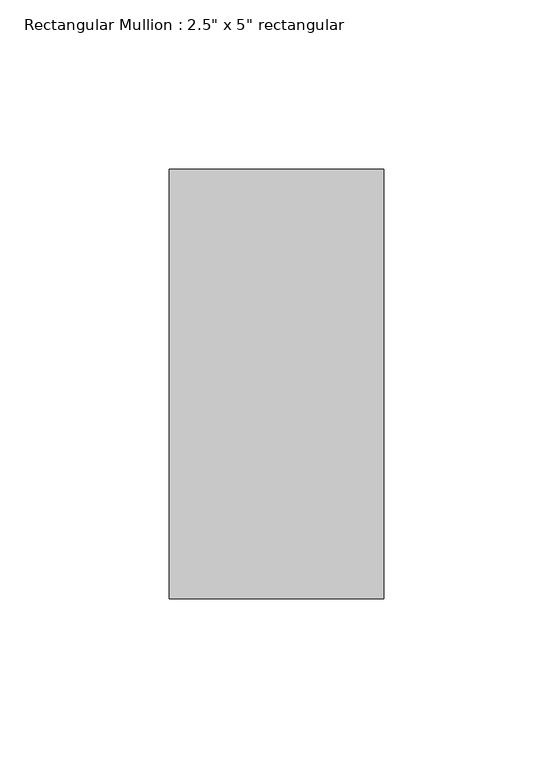
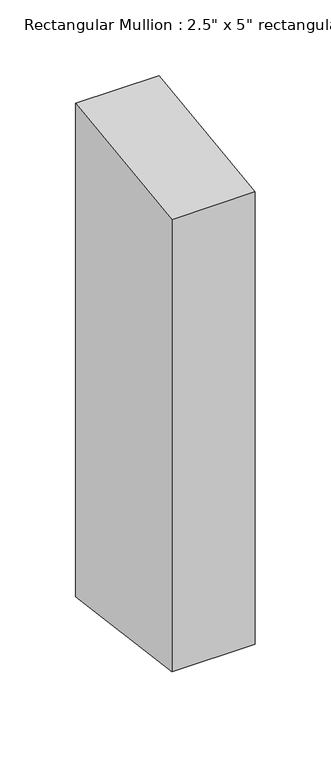
"""IFC4 building model written with IfcOpenShell, lengths in millimetres: member geometry."""

from ifc_helpers import new_model, si_unit, frame, origin, place, context, project, spatial, polyline, outline, extrude, source, transform, mapped, element, save


def member_1e511d5c(model_context):
    return source(origin(), model_context, "Body", "SweptSolid", [
        extrude(outline(polyline([(-63.5, -8.2335242), (63.5, 8.2335242), (63.5, -388.8541629), (-63.5, -372.3871146), (-63.5, -8.2335242)])), frame((-63.5, 0.0, 0.0), z_axis=(1.0, 0.0, 0.0), x_axis=(0.0, 1.0, 0.0)), (0.0, 0.0, 1.0), 63.5),
    ])


if __name__ == "__main__":
    model = new_model("IFC4")
    model_context = context("Model", 3, world=origin())
    ifc_project = project(units=[si_unit("LENGTHUNIT", "METRE", prefix="MILLI")], contexts=[model_context])
    site = spatial("IfcSite", under=ifc_project)
    building = spatial("IfcBuilding", under=site)
    placement = place(None, origin())
    member_shape = member_1e511d5c(model_context)
    element("IfcMember", 1, ObjectType="Rectangular Mullion : 2.5\" x 5\" rectangular", at=placement, inside=building, context=model_context, shape_type="MappedRepresentation", body=[
        mapped(member_shape, transform((0.0, 0.0, 0.0), x_axis=(1.0, 0.0, 0.0), y_axis=(0.0, 1.0, 0.0), z_axis=(0.0, 0.0, 1.0))),
    ])
    save(model, "model.ifc")

# Revit data of these elements
# Type "Rectangular Mullion : 2.5\" x 5\" rectangular"
#   built-in parameter 1007304 = 0.416667 (stored number, unit not read)
#   built-in parameter 1007301 = 0.104167 (stored number, unit not read)
#   built-in parameter 1007300 = 0.104167 (stored number, unit not read)
# Element 1 (IfcMember, "Rectangular Mullion : 2.5\" x 5\" rectangular")
#   Materials on its faces: "Iron, Ductile"
# Materials
#   "Iron, Ductile": class "Metal", colour RGB 0 0 0, transparency 0, Description = "Ductile cast iron", Cost = 0
